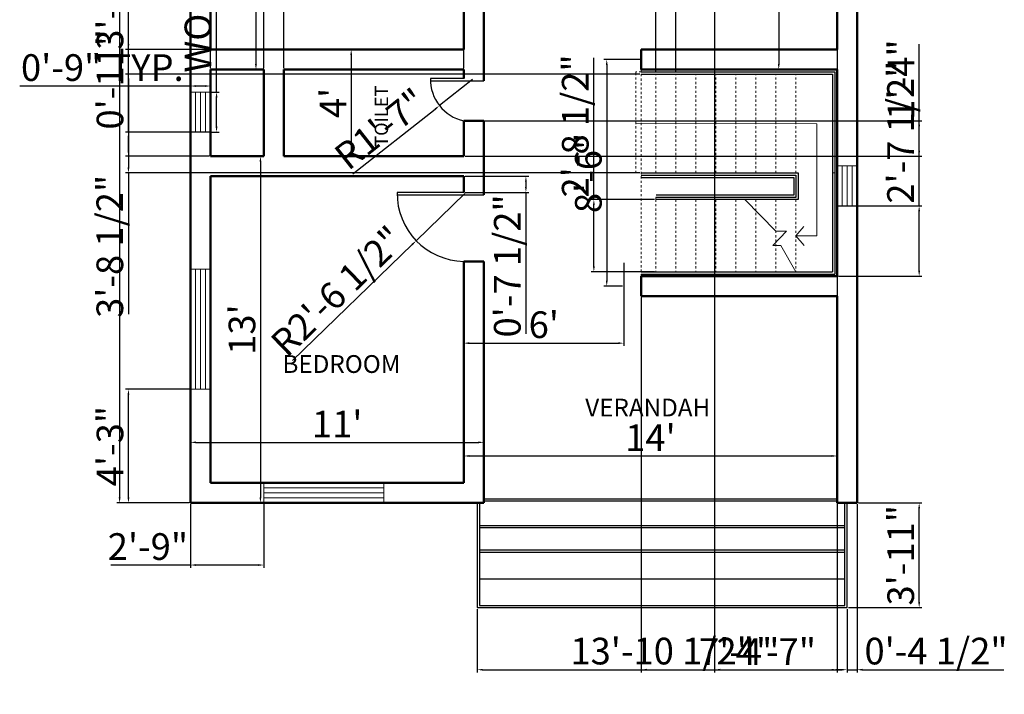
# Model space of a CAD drawing. Units: inches. Extents: x 2490 to 3058, y 1708 to 2351.
# Tile 1 of 2: x 2490 to 2933, y 1708 to 2012. Entities that reach past the tile are written whole.
import ezdxf

# ---------------------------------------------------------------- set-up
doc = ezdxf.new("R2010")
doc.units = ezdxf.units.IN
doc.linetypes.add('JIS_02_1.0', pattern=[2, 1, -1])
for name, color, linetype, lineweight in [('A-ANNO-DIMS', 2, 'Continuous', 18), ('A-ANNO-SYMB', 7, 'Continuous', 18), ('A-AREA-IDEN', 7, 'Continuous', 25), ('A-DOOR', 3, 'Continuous', 25), ('A-FLOR-STRS', 7, 'Continuous', 25), ('A-FLOR-STRS-OVHD', 8, 'JIS_02_1.0', 18), ('A-GLAZ', 4, 'Continuous', 18), ('A-WALL', 7, 'Continuous', 50)]:
    doc.layers.add(name, color=color, linetype=linetype, lineweight=lineweight)
doc.styles.get("Standard").update_dxf_attribs({"font": 'arial.ttf'})
doc.dimstyles.new('ISO-25', dxfattribs={"dimtxt": 12, "dimasz": 2.5, "dimexe": 1.25, "dimexo": 0.625, "dimtad": 1, "dimdec": 1, "dimlunit": 3, "dimtxsty": 'Standard', "dimcen": 2.5, "dimadec": 0, "dimazin": 0, "dimtfac": 1, "dimtdec": 1, "dimtmove": 0, "dimatfit": 3, "dimfxl": 1, "dimarcsym": 0})

# ---------------------------------------------------------------- blocks, each defined once
blk = doc.blocks.new('*D7')
at = {"layer": 'A-ANNO-DIMS', "color": 0, "lineweight": -2, "transparency": 16777216}
for p, q in [((2597.25, 2121.57), (2595.04, 2121.57)), ((2596.29, 2119.07), (2596.29, 1992.07)), ((2597.25, 1989.57), (2595.04, 1989.57))]:
    blk.add_line(p, q, dxfattribs=at)
at = {"layer": 'A-ANNO-DIMS', "color": 0, "transparency": 16777216}
for points in [[(2595.88, 2119.07), (2596.71, 2119.07), (2596.29, 2121.57)], [(2595.88, 1992.07), (2596.71, 1992.07), (2596.29, 1989.57)]]:
    blk.add_solid(points, dxfattribs=at)
at = {"layer": 'Defpoints', "color": 0, "transparency": 16777216}
for p in [(2597.88, 2121.57), (2596.29, 1989.57), (2597.88, 1989.57)]:
    blk.add_point(p, dxfattribs=at)
at = {"layer": 'A-ANNO-DIMS', "color": 0, "transparency": 16777216, "insert": (2589.64, 2055.57), "char_height": 12, "attachment_point": 5, "rotation": 90}
blk.add_mtext("11'", dxfattribs=at)
blk = doc.blocks.new('*D9')
at = {"layer": 'A-ANNO-DIMS', "color": 0, "lineweight": -2, "transparency": 16777216}
for p, q in [((2609.47, 1998.57), (2640.41, 1998.57)), ((2639.16, 1996.07), (2639.16, 1953.07)), ((2609.47, 1950.57), (2640.41, 1950.57))]:
    blk.add_line(p, q, dxfattribs=at)
at = {"layer": 'A-ANNO-DIMS', "color": 0, "transparency": 16777216}
for points in [[(2638.75, 1996.07), (2639.58, 1996.07), (2639.16, 1998.57)], [(2638.75, 1953.07), (2639.58, 1953.07), (2639.16, 1950.57)]]:
    blk.add_solid(points, dxfattribs=at)
at = {"layer": 'Defpoints', "color": 0, "transparency": 16777216}
for p in [(2608.85, 1998.57), (2608.85, 1950.57), (2639.16, 1950.57)]:
    blk.add_point(p, dxfattribs=at)
at = {"layer": 'A-ANNO-DIMS', "color": 0, "transparency": 16777216, "insert": (2632.54, 1974.57), "char_height": 12, "attachment_point": 5, "rotation": 90}
blk.add_mtext("4'", dxfattribs=at)
blk = doc.blocks.new('*D10')
at = {"layer": 'A-ANNO-DIMS', "color": 0, "lineweight": -2, "transparency": 16777216}
for p, q in [((2599.22, 1950.57), (2597.06, 1950.57)), ((2598.31, 1948.07), (2598.31, 1797.07)), ((2599.22, 1794.57), (2597.06, 1794.57))]:
    blk.add_line(p, q, dxfattribs=at)
at = {"layer": 'A-ANNO-DIMS', "color": 0, "transparency": 16777216}
for points in [[(2597.89, 1948.07), (2598.72, 1948.07), (2598.31, 1950.57)], [(2597.89, 1797.07), (2598.72, 1797.07), (2598.31, 1794.57)]]:
    blk.add_solid(points, dxfattribs=at)
at = {"layer": 'Defpoints', "color": 0, "transparency": 16777216}
for p in [(2599.85, 1950.57), (2598.31, 1794.57), (2599.85, 1794.57)]:
    blk.add_point(p, dxfattribs=at)
at = {"layer": 'A-ANNO-DIMS', "color": 0, "transparency": 16777216, "insert": (2591.55, 1872.57), "char_height": 12, "attachment_point": 5, "rotation": 90}
blk.add_mtext("13'", dxfattribs=at)
blk = doc.blocks.new('*D11')
at = {"layer": 'A-ANNO-DIMS', "color": 0, "lineweight": -2, "transparency": 16777216}
for p, q in [((2566.85, 1795.2), (2566.85, 1823.06)), ((2569.35, 1821.81), (2696.35, 1821.81)), ((2698.85, 1795.2), (2698.85, 1823.06))]:
    blk.add_line(p, q, dxfattribs=at)
at = {"layer": 'A-ANNO-DIMS', "color": 0, "transparency": 16777216}
for points in [[(2569.35, 1822.23), (2569.35, 1821.4), (2566.85, 1821.81)], [(2696.35, 1822.23), (2696.35, 1821.4), (2698.85, 1821.81)]]:
    blk.add_solid(points, dxfattribs=at)
at = {"layer": 'Defpoints', "color": 0, "transparency": 16777216}
for p in [(2698.85, 1821.81), (2566.85, 1794.57), (2698.85, 1794.57)]:
    blk.add_point(p, dxfattribs=at)
at = {"layer": 'A-ANNO-DIMS', "color": 0, "transparency": 16777216, "insert": (2632.85, 1828.46), "char_height": 12, "attachment_point": 5}
blk.add_mtext("11'", dxfattribs=at)
blk = doc.blocks.new('*D12')
at = {"layer": 'A-ANNO-DIMS', "color": 0, "lineweight": -2, "transparency": 16777216}
for p, q in [((2769.12, 1994.07), (2752.94, 1994.07)), ((2754.19, 1991.57), (2754.19, 1894.57)), ((2761.22, 1892.07), (2752.94, 1892.07))]:
    blk.add_line(p, q, dxfattribs=at)
at = {"layer": 'A-ANNO-DIMS', "color": 0, "transparency": 16777216}
for points in [[(2753.77, 1991.57), (2754.6, 1991.57), (2754.19, 1994.07)], [(2753.77, 1894.57), (2754.6, 1894.57), (2754.19, 1892.07)]]:
    blk.add_solid(points, dxfattribs=at)
at = {"layer": 'Defpoints', "color": 0, "transparency": 16777216}
for p in [(2769.74, 1994.07), (2754.19, 1892.07), (2761.85, 1892.07)]:
    blk.add_point(p, dxfattribs=at)
at = {"layer": 'A-ANNO-DIMS', "color": 0, "transparency": 16777216, "insert": (2747.43, 1943.07), "char_height": 12, "attachment_point": 5, "rotation": 90}
blk.add_mtext('8\'-6"', dxfattribs=at)
blk = doc.blocks.new('*D13')
at = {"layer": 'A-ANNO-DIMS', "color": 0, "lineweight": -2, "transparency": 16777216}
for p, q in [((2689.85, 1902.66), (2689.85, 1865.21)), ((2761.85, 1902.66), (2761.85, 1865.21)), ((2692.35, 1866.46), (2759.35, 1866.46))]:
    blk.add_line(p, q, dxfattribs=at)
at = {"layer": 'A-ANNO-DIMS', "color": 0, "transparency": 16777216}
for points in [[(2692.35, 1866.88), (2692.35, 1866.04), (2689.85, 1866.46)], [(2759.35, 1866.88), (2759.35, 1866.04), (2761.85, 1866.46)]]:
    blk.add_solid(points, dxfattribs=at)
at = {"layer": 'Defpoints', "color": 0, "transparency": 16777216}
for p in [(2689.85, 1903.28), (2761.85, 1903.28), (2761.85, 1866.46)]:
    blk.add_point(p, dxfattribs=at)
at = {"layer": 'A-ANNO-DIMS', "color": 0, "transparency": 16777216, "insert": (2725.85, 1873.21), "char_height": 12, "attachment_point": 5}
blk.add_mtext("6'", dxfattribs=at)
blk = doc.blocks.new('*D14')
at = {"layer": 'A-ANNO-DIMS', "color": 0, "lineweight": -2, "transparency": 16777216}
for p, q in [((2847.51, 2169.63), (2830.36, 2169.63)), ((2831.61, 2167.13), (2831.61, 1992.13)), ((2847.51, 1989.63), (2830.36, 1989.63))]:
    blk.add_line(p, q, dxfattribs=at)
at = {"layer": 'A-ANNO-DIMS', "color": 0, "transparency": 16777216}
for points in [[(2831.19, 2167.13), (2832.02, 2167.13), (2831.61, 2169.63)], [(2831.19, 1992.13), (2832.02, 1992.13), (2831.61, 1989.63)]]:
    blk.add_solid(points, dxfattribs=at)
at = {"layer": 'Defpoints', "color": 0, "transparency": 16777216}
for p in [(2848.13, 2169.63), (2831.61, 1989.63), (2848.13, 1989.63)]:
    blk.add_point(p, dxfattribs=at)
at = {"layer": 'A-ANNO-DIMS', "color": 0, "transparency": 16777216, "insert": (2824.86, 2079.63), "char_height": 12, "attachment_point": 5, "rotation": 90}
blk.add_mtext("15'", dxfattribs=at)
blk = doc.blocks.new('*D16')
at = {"layer": 'A-ANNO-DIMS', "color": 0, "lineweight": -2, "transparency": 16777216}
for p, q in [((2689.85, 1804.2), (2689.85, 1816.94)), ((2692.35, 1815.69), (2855.35, 1815.69)), ((2857.85, 1804.2), (2857.85, 1816.94))]:
    blk.add_line(p, q, dxfattribs=at)
at = {"layer": 'A-ANNO-DIMS', "color": 0, "transparency": 16777216}
for points in [[(2692.35, 1816.11), (2692.35, 1815.28), (2689.85, 1815.69)], [(2855.35, 1816.11), (2855.35, 1815.28), (2857.85, 1815.69)]]:
    blk.add_solid(points, dxfattribs=at)
at = {"layer": 'Defpoints', "color": 0, "transparency": 16777216}
for p in [(2857.85, 1815.69), (2689.85, 1803.57), (2857.85, 1803.57)]:
    blk.add_point(p, dxfattribs=at)
at = {"layer": 'A-ANNO-DIMS', "color": 0, "transparency": 16777216, "insert": (2773.85, 1822.34), "char_height": 12, "attachment_point": 5}
blk.add_mtext("14'", dxfattribs=at)
blk = doc.blocks.new('Window - Wood Frame 36 in. Wide plan')
for p, q in [((0, 6), (0, 0)), ((36, 6), (36, 0)), ((0, 4.5), (36, 4.5)), ((0, 3), (36, 3)), ((0, 1.5), (36, 1.5))]:
    blk.add_line(p, q)
blk = doc.blocks.new('*D22')
at = {"layer": 'A-ANNO-DIMS', "color": 0, "lineweight": -2, "transparency": 16777216}
for p, q in [((2566.22, 2274.57), (2533.68, 2274.57)), ((2534.93, 2272.07), (2534.93, 1797.07)), ((2566.22, 1794.57), (2533.68, 1794.57))]:
    blk.add_line(p, q, dxfattribs=at)
at = {"layer": 'A-ANNO-DIMS', "color": 0, "transparency": 16777216}
for points in [[(2534.51, 2272.07), (2535.35, 2272.07), (2534.93, 2274.57)], [(2534.51, 1797.07), (2535.35, 1797.07), (2534.93, 1794.57)]]:
    blk.add_solid(points, dxfattribs=at)
at = {"layer": 'Defpoints', "color": 0, "transparency": 16777216}
for p in [(2566.85, 2274.57), (2534.93, 1794.57), (2566.85, 1794.57)]:
    blk.add_point(p, dxfattribs=at)
at = {"layer": 'A-ANNO-DIMS', "color": 0, "transparency": 16777216, "insert": (2528.18, 2034.57), "char_height": 12, "attachment_point": 5, "rotation": 90}
blk.add_mtext("40'", dxfattribs=at)
blk = doc.blocks.new('*D26')
at = {"layer": 'A-ANNO-DIMS', "color": 0, "lineweight": -2, "transparency": 16777216}
for p, q in [((2578.55, 1979.48), (2578.55, 2193.75)), ((2576.47, 1979.48), (2579.8, 1979.48)), ((2578.55, 1963.98), (2578.55, 1976.98)), ((2576.47, 1961.48), (2579.8, 1961.48))]:
    blk.add_line(p, q, dxfattribs=at)
at = {"layer": 'A-ANNO-DIMS', "color": 0, "transparency": 16777216}
for points in [[(2578.13, 1976.98), (2578.97, 1976.98), (2578.55, 1979.48)], [(2578.13, 1963.98), (2578.97, 1963.98), (2578.55, 1961.48)]]:
    blk.add_solid(points, dxfattribs=at)
at = {"layer": 'Defpoints', "color": 0, "transparency": 16777216}
for p in [(2575.85, 1979.48), (2578.55, 1979.48), (2575.85, 1961.48)]:
    blk.add_point(p, dxfattribs=at)
at = {"layer": 'A-ANNO-DIMS', "color": 0, "transparency": 16777216, "insert": (2571.72, 2087.86), "char_height": 12, "attachment_point": 5, "rotation": 90}
blk.add_mtext('WOOD WINDOW 1\'-6" TYP.', dxfattribs=at)
blk = doc.blocks.new('*D27')
at = {"layer": 'A-ANNO-DIMS', "color": 0, "lineweight": -2, "transparency": 16777216}
for p, q in [((2566.85, 1982.18), (2489.95, 1982.18)), ((2566.85, 1980.11), (2566.85, 1983.43)), ((2573.35, 1982.18), (2569.35, 1982.18)), ((2575.85, 1980.11), (2575.85, 1983.43))]:
    blk.add_line(p, q, dxfattribs=at)
at = {"layer": 'A-ANNO-DIMS', "color": 0, "transparency": 16777216}
for points in [[(2569.35, 1982.6), (2569.35, 1981.76), (2566.85, 1982.18)], [(2573.35, 1982.6), (2573.35, 1981.76), (2575.85, 1982.18)]]:
    blk.add_solid(points, dxfattribs=at)
at = {"layer": 'Defpoints', "color": 0, "transparency": 16777216}
for p in [(2566.85, 1982.18), (2566.85, 1979.48), (2575.85, 1979.48)]:
    blk.add_point(p, dxfattribs=at)
at = {"layer": 'A-ANNO-DIMS', "color": 0, "transparency": 16777216, "insert": (2527.15, 1988.93), "char_height": 12, "attachment_point": 5}
blk.add_mtext('0\'-9" TYP.', dxfattribs=at)
blk = doc.blocks.new('*D30')
at = {"layer": 'A-ANNO-DIMS', "color": 0, "lineweight": -2, "transparency": 16777216}
for p, q in [((2695.91, 1746.82), (2695.91, 1718.25)), ((2862.35, 1746.82), (2862.35, 1718.25)), ((2698.41, 1719.5), (2859.85, 1719.5))]:
    blk.add_line(p, q, dxfattribs=at)
at = {"layer": 'A-ANNO-DIMS', "color": 0, "transparency": 16777216}
for points in [[(2698.41, 1719.92), (2698.41, 1719.08), (2695.91, 1719.5)], [(2859.85, 1719.92), (2859.85, 1719.08), (2862.35, 1719.5)]]:
    blk.add_solid(points, dxfattribs=at)
at = {"layer": 'Defpoints', "color": 0, "transparency": 16777216}
for p in [(2695.91, 1747.45), (2862.35, 1747.45), (2862.35, 1719.5)]:
    blk.add_point(p, dxfattribs=at)
at = {"layer": 'A-ANNO-DIMS', "color": 0, "transparency": 16777216, "insert": (2779.13, 1726.33), "char_height": 12, "attachment_point": 5}
blk.add_mtext('13\'-10 1/2"', dxfattribs=at)
blk = doc.blocks.new('*D31')
at = {"layer": 'A-ANNO-DIMS', "color": 0, "lineweight": -2, "transparency": 16777216}
for p, q in [((2867.47, 1794.57), (2896.05, 1794.57)), ((2894.8, 1749.95), (2894.8, 1792.07)), ((2862.97, 1747.45), (2896.05, 1747.45))]:
    blk.add_line(p, q, dxfattribs=at)
at = {"layer": 'A-ANNO-DIMS', "color": 0, "transparency": 16777216}
for points in [[(2894.38, 1792.07), (2895.22, 1792.07), (2894.8, 1794.57)], [(2894.38, 1749.95), (2895.22, 1749.95), (2894.8, 1747.45)]]:
    blk.add_solid(points, dxfattribs=at)
at = {"layer": 'Defpoints', "color": 0, "transparency": 16777216}
for p in [(2866.85, 1794.57), (2894.8, 1794.57), (2862.35, 1747.45)]:
    blk.add_point(p, dxfattribs=at)
at = {"layer": 'A-ANNO-DIMS', "color": 0, "transparency": 16777216, "insert": (2888.04, 1771.01), "char_height": 12, "attachment_point": 5, "rotation": 90}
blk.add_mtext('3\'-11"', dxfattribs=at)
blk = doc.blocks.new('*D32')
at = {"layer": 'A-ANNO-DIMS', "color": 0, "lineweight": -2, "transparency": 16777216}
for p, q in [((2769.74, 1886.95), (2769.74, 1718.25)), ((2857.85, 1886.95), (2857.85, 1718.25)), ((2772.24, 1719.5), (2855.35, 1719.5))]:
    blk.add_line(p, q, dxfattribs=at)
at = {"layer": 'A-ANNO-DIMS', "color": 0, "transparency": 16777216}
for points in [[(2772.24, 1719.92), (2772.24, 1719.08), (2769.74, 1719.5)], [(2855.35, 1719.92), (2855.35, 1719.08), (2857.85, 1719.5)]]:
    blk.add_solid(points, dxfattribs=at)
at = {"layer": 'Defpoints', "color": 0, "transparency": 16777216}
for p in [(2769.74, 1887.57), (2857.85, 1887.57), (2857.85, 1719.5)]:
    blk.add_point(p, dxfattribs=at)
at = {"layer": 'A-ANNO-DIMS', "color": 0, "transparency": 16777216, "insert": (2813.8, 1726.12), "char_height": 12, "attachment_point": 5}
blk.add_mtext('7\'-4"', dxfattribs=at)
blk = doc.blocks.new('*D33')
at = {"layer": 'A-ANNO-DIMS', "color": 0, "lineweight": -2, "transparency": 16777216}
for p, q in [((2608.85, 1990.2), (2608.85, 2303.77)), ((2611.35, 2302.52), (2687.35, 2302.52)), ((2689.85, 1990.2), (2689.85, 2303.77))]:
    blk.add_line(p, q, dxfattribs=at)
at = {"layer": 'A-ANNO-DIMS', "color": 0, "transparency": 16777216}
for points in [[(2611.35, 2302.94), (2611.35, 2302.1), (2608.85, 2302.52)], [(2687.35, 2302.94), (2687.35, 2302.1), (2689.85, 2302.52)]]:
    blk.add_solid(points, dxfattribs=at)
at = {"layer": 'Defpoints', "color": 0, "transparency": 16777216}
for p in [(2689.85, 2302.52), (2608.85, 1989.57), (2689.85, 1989.57)]:
    blk.add_point(p, dxfattribs=at)
at = {"layer": 'A-ANNO-DIMS', "color": 0, "transparency": 16777216, "insert": (2649.35, 2309.27), "char_height": 12, "attachment_point": 5}
blk.add_mtext('6\'-9"', dxfattribs=at)
blk = doc.blocks.new('*D36')
at = {"layer": 'A-ANNO-DIMS', "color": 0, "lineweight": -2, "transparency": 16777216}
for p, q in [((2802.74, 2168.95), (2802.74, 1718.25)), ((2857.85, 2168.95), (2857.85, 1718.25)), ((2805.24, 1719.5), (2855.35, 1719.5))]:
    blk.add_line(p, q, dxfattribs=at)
at = {"layer": 'A-ANNO-DIMS', "color": 0, "transparency": 16777216}
for points in [[(2805.24, 1719.92), (2805.24, 1719.08), (2802.74, 1719.5)], [(2855.35, 1719.92), (2855.35, 1719.08), (2857.85, 1719.5)]]:
    blk.add_solid(points, dxfattribs=at)
at = {"layer": 'Defpoints', "color": 0, "transparency": 16777216}
for p in [(2802.74, 2169.57), (2857.85, 2169.57), (2857.85, 1719.5)]:
    blk.add_point(p, dxfattribs=at)
at = {"layer": 'A-ANNO-DIMS', "color": 0, "transparency": 16777216, "insert": (2830.3, 1726.12), "char_height": 12, "attachment_point": 5}
blk.add_mtext('4\'-7"', dxfattribs=at)
blk = doc.blocks.new('*D38')
at = {"layer": 'A-ANNO-DIMS', "color": 0, "lineweight": -2, "transparency": 16777216}
for p, q in [((2894.8, 1966.57), (2894.8, 2001.09)), ((2690.47, 1966.57), (2896.05, 1966.57)), ((2894.8, 1953.07), (2894.8, 1964.07)), ((2690.47, 1950.57), (2896.05, 1950.57))]:
    blk.add_line(p, q, dxfattribs=at)
at = {"layer": 'A-ANNO-DIMS', "color": 0, "transparency": 16777216}
for points in [[(2894.38, 1964.07), (2895.22, 1964.07), (2894.8, 1966.57)], [(2894.38, 1953.07), (2895.22, 1953.07), (2894.8, 1950.57)]]:
    blk.add_solid(points, dxfattribs=at)
at = {"layer": 'Defpoints', "color": 0, "transparency": 16777216}
for p in [(2689.85, 1966.57), (2894.8, 1966.57), (2689.85, 1950.57)]:
    blk.add_point(p, dxfattribs=at)
at = {"layer": 'A-ANNO-DIMS', "color": 0, "transparency": 16777216, "insert": (2888.15, 1985.08), "char_height": 12, "attachment_point": 5, "rotation": 90}
blk.add_mtext('1\'-4"', dxfattribs=at)
blk = doc.blocks.new('*D39')
at = {"layer": 'A-ANNO-DIMS', "color": 0, "lineweight": -2, "transparency": 16777216}
for p, q in [((2538.9, 1961.48), (2538.9, 2006.45)), ((2575.22, 1961.48), (2537.65, 1961.48)), ((2538.9, 1953.07), (2538.9, 1958.98)), ((2575.22, 1950.57), (2537.65, 1950.57))]:
    blk.add_line(p, q, dxfattribs=at)
at = {"layer": 'A-ANNO-DIMS', "color": 0, "transparency": 16777216}
for points in [[(2538.48, 1958.98), (2539.32, 1958.98), (2538.9, 1961.48)], [(2538.48, 1953.07), (2539.32, 1953.07), (2538.9, 1950.57)]]:
    blk.add_solid(points, dxfattribs=at)
at = {"layer": 'Defpoints', "color": 0, "transparency": 16777216}
for p in [(2538.9, 1961.48), (2575.85, 1961.48), (2575.85, 1950.57)]:
    blk.add_point(p, dxfattribs=at)
at = {"layer": 'A-ANNO-DIMS', "color": 0, "transparency": 16777216, "insert": (2532.15, 1985.22), "char_height": 12, "attachment_point": 5, "rotation": 90}
blk.add_mtext('0\'-11"', dxfattribs=at)
blk = doc.blocks.new('*D40')
at = {"layer": 'A-ANNO-DIMS', "color": 0, "lineweight": -2, "transparency": 16777216}
for p, q in [((2575.85, 1990.2), (2575.85, 2303.77)), ((2578.35, 2302.52), (2597.35, 2302.52)), ((2599.85, 1990.2), (2599.85, 2303.77)), ((2599.85, 2302.52), (2635.7, 2302.52))]:
    blk.add_line(p, q, dxfattribs=at)
at = {"layer": 'A-ANNO-DIMS', "color": 0, "transparency": 16777216}
for points in [[(2578.35, 2302.94), (2578.35, 2302.1), (2575.85, 2302.52)], [(2597.35, 2302.94), (2597.35, 2302.1), (2599.85, 2302.52)]]:
    blk.add_solid(points, dxfattribs=at)
at = {"layer": 'Defpoints', "color": 0, "transparency": 16777216}
for p in [(2599.85, 2302.52), (2575.85, 1989.57), (2599.85, 1989.57)]:
    blk.add_point(p, dxfattribs=at)
at = {"layer": 'A-ANNO-DIMS', "color": 0, "transparency": 16777216, "insert": (2619.03, 2309.27), "char_height": 12, "attachment_point": 5}
blk.add_mtext('2\'-0"', dxfattribs=at)
blk = doc.blocks.new('*D43')
at = {"layer": 'A-ANNO-DIMS', "color": 0, "lineweight": -2, "transparency": 16777216}
for p, q in [((2575.22, 2034.57), (2537.65, 2034.57)), ((2538.9, 2001.07), (2538.9, 2032.07)), ((2575.22, 1998.57), (2537.65, 1998.57))]:
    blk.add_line(p, q, dxfattribs=at)
at = {"layer": 'A-ANNO-DIMS', "color": 0, "transparency": 16777216}
for points in [[(2538.48, 2032.07), (2539.32, 2032.07), (2538.9, 2034.57)], [(2538.48, 2001.07), (2539.32, 2001.07), (2538.9, 1998.57)]]:
    blk.add_solid(points, dxfattribs=at)
at = {"layer": 'Defpoints', "color": 0, "transparency": 16777216}
for p in [(2538.9, 2034.57), (2575.85, 2034.57), (2575.85, 1998.57)]:
    blk.add_point(p, dxfattribs=at)
at = {"layer": 'A-ANNO-DIMS', "color": 0, "transparency": 16777216, "insert": (2532.14, 2016.57), "char_height": 12, "attachment_point": 5, "rotation": 90}
blk.add_mtext('3\'-0"', dxfattribs=at)
blk = doc.blocks.new('*D44')
at = {"layer": 'A-ANNO-DIMS', "color": 0, "lineweight": -2, "transparency": 16777216}
for p, q in [((2566.22, 1845.71), (2537.65, 1845.71)), ((2538.9, 1797.07), (2538.9, 1843.21)), ((2566.22, 1794.57), (2537.65, 1794.57))]:
    blk.add_line(p, q, dxfattribs=at)
at = {"layer": 'A-ANNO-DIMS', "color": 0, "transparency": 16777216}
for points in [[(2538.48, 1843.21), (2539.32, 1843.21), (2538.9, 1845.71)], [(2538.48, 1797.07), (2539.32, 1797.07), (2538.9, 1794.57)]]:
    blk.add_solid(points, dxfattribs=at)
at = {"layer": 'Defpoints', "color": 0, "transparency": 16777216}
for p in [(2538.9, 1845.71), (2566.85, 1845.71), (2566.85, 1794.57)]:
    blk.add_point(p, dxfattribs=at)
at = {"layer": 'A-ANNO-DIMS', "color": 0, "transparency": 16777216, "insert": (2532.14, 1820.14), "char_height": 12, "attachment_point": 5, "rotation": 90}
blk.add_mtext('4\'-3"', dxfattribs=at)
blk = doc.blocks.new('*D45')
at = {"layer": 'A-ANNO-DIMS', "color": 0, "lineweight": -2, "transparency": 16777216}
for p, q in [((2566.85, 1793.95), (2566.85, 1765.37)), ((2599.85, 1793.95), (2599.85, 1765.37)), ((2566.85, 1766.62), (2531, 1766.62)), ((2597.35, 1766.62), (2569.35, 1766.62))]:
    blk.add_line(p, q, dxfattribs=at)
at = {"layer": 'A-ANNO-DIMS', "color": 0, "transparency": 16777216}
for points in [[(2569.35, 1767.04), (2569.35, 1766.2), (2566.85, 1766.62)], [(2597.35, 1767.04), (2597.35, 1766.2), (2599.85, 1766.62)]]:
    blk.add_solid(points, dxfattribs=at)
at = {"layer": 'Defpoints', "color": 0, "transparency": 16777216}
for p in [(2566.85, 1794.57), (2599.85, 1794.57), (2566.85, 1766.62)]:
    blk.add_point(p, dxfattribs=at)
at = {"layer": 'A-ANNO-DIMS', "color": 0, "transparency": 16777216, "insert": (2547.67, 1773.37), "char_height": 12, "attachment_point": 5}
blk.add_mtext('2\'-9"', dxfattribs=at)
blk = doc.blocks.new('*D47')
at = {"layer": 'A-ANNO-DIMS', "color": 0, "lineweight": -2, "transparency": 16777216}
for p, q in [((2894.8, 1928.26), (2894.8, 1992.08)), ((2858.47, 1928.26), (2896.05, 1928.26)), ((2894.8, 1899.07), (2894.8, 1925.76)), ((2858.47, 1896.57), (2896.05, 1896.57))]:
    blk.add_line(p, q, dxfattribs=at)
at = {"layer": 'A-ANNO-DIMS', "color": 0, "transparency": 16777216}
for points in [[(2894.38, 1925.76), (2895.22, 1925.76), (2894.8, 1928.26)], [(2894.38, 1899.07), (2895.22, 1899.07), (2894.8, 1896.57)]]:
    blk.add_solid(points, dxfattribs=at)
at = {"layer": 'Defpoints', "color": 0, "transparency": 16777216}
for p in [(2857.85, 1928.26), (2894.8, 1928.26), (2857.85, 1896.57)]:
    blk.add_point(p, dxfattribs=at)
at = {"layer": 'A-ANNO-DIMS', "color": 0, "transparency": 16777216, "insert": (2887.97, 1961.42), "char_height": 12, "attachment_point": 5, "rotation": 90}
blk.add_mtext('2\'-7 1/2"', dxfattribs=at)
blk = doc.blocks.new('*D50')
at = {"layer": 'A-ANNO-DIMS', "color": 0, "lineweight": -2, "transparency": 16777216}
for p, q in [((2690.47, 1941.57), (2719.05, 1941.57)), ((2717.8, 1939.07), (2717.8, 1936.78)), ((2690.47, 1934.28), (2719.05, 1934.28)), ((2717.8, 1934.28), (2717.8, 1870.67))]:
    blk.add_line(p, q, dxfattribs=at)
at = {"layer": 'A-ANNO-DIMS', "color": 0, "transparency": 16777216}
for points in [[(2717.38, 1939.07), (2718.22, 1939.07), (2717.8, 1941.57)], [(2717.38, 1936.78), (2718.22, 1936.78), (2717.8, 1934.28)]]:
    blk.add_solid(points, dxfattribs=at)
at = {"layer": 'Defpoints', "color": 0, "transparency": 16777216}
for p in [(2689.85, 1941.57), (2689.85, 1934.28), (2717.8, 1934.28)]:
    blk.add_point(p, dxfattribs=at)
at = {"layer": 'A-ANNO-DIMS', "color": 0, "transparency": 16777216, "insert": (2710.97, 1901.23), "char_height": 12, "attachment_point": 5, "rotation": 90}
blk.add_mtext('0\'-7 1/2"', dxfattribs=at)
blk = doc.blocks.new('*D51')
at = {"layer": 'A-ANNO-DIMS', "color": 0, "lineweight": -2, "transparency": 16777216}
for p, q in [((2776.33, 1988.2), (2776.33, 2303.77)), ((2778.83, 2302.52), (2782.83, 2302.52)), ((2785.33, 1988.2), (2785.33, 2303.77)), ((2785.33, 2302.52), (2820.98, 2302.52))]:
    blk.add_line(p, q, dxfattribs=at)
at = {"layer": 'A-ANNO-DIMS', "color": 0, "transparency": 16777216}
for points in [[(2778.83, 2302.94), (2778.83, 2302.1), (2776.33, 2302.52)], [(2782.83, 2302.94), (2782.83, 2302.1), (2785.33, 2302.52)]]:
    blk.add_solid(points, dxfattribs=at)
at = {"layer": 'Defpoints', "color": 0, "transparency": 16777216}
for p in [(2785.33, 2302.52), (2776.33, 1987.57), (2785.33, 1987.57)]:
    blk.add_point(p, dxfattribs=at)
at = {"layer": 'A-ANNO-DIMS', "color": 0, "transparency": 16777216, "insert": (2804.41, 2309.27), "char_height": 12, "attachment_point": 5}
blk.add_mtext('0\'-9"', dxfattribs=at)
blk = doc.blocks.new('*D52')
at = {"layer": 'A-ANNO-DIMS', "color": 0, "lineweight": -2, "transparency": 16777216}
for p, q in [((2769.12, 1987.57), (2537.65, 1987.57)), ((2538.9, 1985.07), (2538.9, 1945.57)), ((2769.12, 1943.07), (2537.65, 1943.07)), ((2538.9, 1943.07), (2538.9, 1879.47))]:
    blk.add_line(p, q, dxfattribs=at)
at = {"layer": 'A-ANNO-DIMS', "color": 0, "transparency": 16777216}
for points in [[(2538.48, 1985.07), (2539.32, 1985.07), (2538.9, 1987.57)], [(2538.48, 1945.57), (2539.32, 1945.57), (2538.9, 1943.07)]]:
    blk.add_solid(points, dxfattribs=at)
at = {"layer": 'Defpoints', "color": 0, "transparency": 16777216}
for p in [(2769.74, 1987.57), (2538.9, 1943.07), (2769.74, 1943.07)]:
    blk.add_point(p, dxfattribs=at)
at = {"layer": 'A-ANNO-DIMS', "color": 0, "transparency": 16777216, "insert": (2532.07, 1910.02), "char_height": 12, "attachment_point": 5, "rotation": 90}
blk.add_mtext('3\'-8 1/2"', dxfattribs=at)
blk = doc.blocks.new('*D53')
at = {"layer": 'A-ANNO-DIMS', "color": 0, "lineweight": -2, "transparency": 16777216}
for p, q in [((2748.38, 1931.07), (2748.38, 1994.89)), ((2775.71, 1931.07), (2747.13, 1931.07)), ((2748.38, 1901.07), (2748.38, 1928.57)), ((2775.71, 1898.57), (2747.13, 1898.57))]:
    blk.add_line(p, q, dxfattribs=at)
at = {"layer": 'A-ANNO-DIMS', "color": 0, "transparency": 16777216}
for points in [[(2747.96, 1928.57), (2748.8, 1928.57), (2748.38, 1931.07)], [(2747.96, 1901.07), (2748.8, 1901.07), (2748.38, 1898.57)]]:
    blk.add_solid(points, dxfattribs=at)
at = {"layer": 'Defpoints', "color": 0, "transparency": 16777216}
for p in [(2748.38, 1931.07), (2776.33, 1931.07), (2776.33, 1898.57)]:
    blk.add_point(p, dxfattribs=at)
at = {"layer": 'A-ANNO-DIMS', "color": 0, "transparency": 16777216, "insert": (2741.55, 1964.23), "char_height": 12, "attachment_point": 5, "rotation": 90}
blk.add_mtext('2\'-8 1/2"', dxfattribs=at)
blk = doc.blocks.new('*D54')
at = {"layer": 'A-ANNO-DIMS', "color": 0, "lineweight": -2, "transparency": 16777216}
for p, q in [((2866.85, 1793.95), (2866.85, 1718.25)), ((2862.35, 1746.82), (2862.35, 1718.25)), ((2859.85, 1719.5), (2857.35, 1719.5)), ((2862.35, 1719.5), (2866.85, 1719.5)), ((2869.35, 1719.5), (2932.96, 1719.5))]:
    blk.add_line(p, q, dxfattribs=at)
at = {"layer": 'A-ANNO-DIMS', "color": 0, "transparency": 16777216}
for points in [[(2859.85, 1719.92), (2859.85, 1719.08), (2862.35, 1719.5)], [(2869.35, 1719.92), (2869.35, 1719.08), (2866.85, 1719.5)]]:
    blk.add_solid(points, dxfattribs=at)
at = {"layer": 'Defpoints', "color": 0, "transparency": 16777216}
for p in [(2866.85, 1794.57), (2862.35, 1747.45), (2866.85, 1719.5)]:
    blk.add_point(p, dxfattribs=at)
at = {"layer": 'A-ANNO-DIMS', "color": 0, "transparency": 16777216, "insert": (2902.4, 1726.33), "char_height": 12, "attachment_point": 5}
blk.add_mtext('0\'-4 1/2"', dxfattribs=at)
blk = doc.blocks.new('*D55')
at = {"layer": 'A-ANNO-DIMS', "color": 0, "lineweight": -2, "transparency": 16777216}
for p, q in [((2690.35, 1933.78), (2668.43, 1912.57)), ((2612.67, 1858.61), (2666.63, 1910.83))]:
    blk.add_line(p, q, dxfattribs=at)
at = {"layer": 'A-ANNO-DIMS', "color": 0, "transparency": 16777216}
blk.add_solid([(2666.34, 1911.13), (2666.92, 1910.53), (2668.43, 1912.57)], dxfattribs=at)
at = {"layer": 'Defpoints', "color": 0, "transparency": 16777216}
for p in [(2690.35, 1933.78), (2668.43, 1912.57)]:
    blk.add_point(p, dxfattribs=at)
at = {"layer": 'A-ANNO-DIMS', "color": 0, "transparency": 16777216, "insert": (2634, 1888.76), "char_height": 12, "attachment_point": 5, "rotation": 44.0613}
blk.add_mtext('R2\'-6 1/2"', dxfattribs=at)
blk = doc.blocks.new('*D60')
at = {"layer": 'A-ANNO-DIMS', "color": 0, "lineweight": -2, "transparency": 16777216}
for p, q in [((2693.75, 1985.07), (2678.91, 1973.36)), ((2639.95, 1942.6), (2676.95, 1971.81))]:
    blk.add_line(p, q, dxfattribs=at)
at = {"layer": 'A-ANNO-DIMS', "color": 0, "transparency": 16777216}
blk.add_solid([(2676.69, 1972.13), (2677.21, 1971.48), (2678.91, 1973.36)], dxfattribs=at)
at = {"layer": 'Defpoints', "color": 0, "transparency": 16777216}
for p in [(2693.75, 1985.07), (2678.91, 1973.36)]:
    blk.add_point(p, dxfattribs=at)
at = {"layer": 'A-ANNO-DIMS', "color": 0, "transparency": 16777216, "insert": (2653.35, 1961.65), "char_height": 12, "attachment_point": 5, "rotation": 38.2892}
blk.add_mtext('R1\'-7"', dxfattribs=at)

msp = doc.modelspace()

# ---------------------------------------------------------------- linework, layer by layer
at = {"layer": 'A-ANNO-SYMB'}
for p, q in [((2767.33, 1965.32), (2848.7, 1965.11)), ((2848.7, 1965.11), (2848.7, 1914.82)), ((2830.33, 1916.81), (2816.33, 1931.07)), ((2828.89, 1910.43), (2835.07, 1916.81)), ((2835.07, 1916.81), (2830.33, 1916.81)), ((2839.33, 1914.82), (2842.85, 1918.92)), ((2848.7, 1914.82), (2839.33, 1914.82)), ((2839.33, 1914.82), (2842.98, 1910.36)), ((2832.49, 1910.43), (2828.89, 1910.43)), ((2839.33, 1898.57), (2832.49, 1910.43))]:
    msp.add_line(p, q, dxfattribs=at)
at = {"layer": 'A-DOOR'}
for p, q in [((2689.85, 1985.57), (2674.85, 1985.57)), ((2674.85, 1985.57), (2674.85, 1984.57)), ((2674.85, 1984.57), (2698.85, 1984.57)), ((2689.85, 1934.28), (2659.85, 1934.28)), ((2659.85, 1934.28), (2659.85, 1933.28)), ((2659.85, 1933.28), (2698.85, 1933.28))]:
    msp.add_line(p, q, dxfattribs=at)
for centre, radius, start, end in [((2693.75, 1985.07), 18.91, 178.4846, 258.0957), ((2690.35, 1933.78), 30.5, 179.0608, 269.0608)]:
    msp.add_arc(centre, radius, start, end, dxfattribs=at)
at = {"layer": 'A-FLOR-STRS'}
for p, q in [((2769.74, 1988.57), (2856.85, 1988.57)), ((2769.74, 1987.57), (2855.85, 1987.57)), ((2855.85, 1987.57), (2855.85, 1898.57)), ((2856.85, 1988.57), (2856.85, 1897.57)), ((2769.74, 1943.07), (2840.33, 1943.07)), ((2769.74, 1942.07), (2839.33, 1942.07)), ((2839.33, 1942.07), (2839.33, 1932.07)), ((2840.33, 1943.07), (2840.33, 1931.07)), ((2769.74, 1941.07), (2838.33, 1941.07)), ((2838.33, 1941.07), (2838.33, 1933.07)), ((2838.33, 1933.07), (2776.5, 1933.07)), ((2839.33, 1932.07), (2776.33, 1932.07)), ((2840.33, 1931.07), (2776.33, 1931.07)), ((2769.74, 1898.57), (2855.85, 1898.57)), ((2769.74, 1897.57), (2856.85, 1897.57)), ((2698.85, 1796.45), (2857.85, 1796.45)), ((2698.85, 1795.45), (2857.85, 1795.45)), ((2695.91, 1794.57), (2695.91, 1747.45)), ((2696.91, 1794.57), (2696.91, 1748.45)), ((2861.35, 1748.45), (2861.35, 1794.57)), ((2862.35, 1747.45), (2862.35, 1794.57)), ((2696.91, 1784.45), (2861.35, 1784.45)), ((2696.91, 1783.45), (2861.35, 1783.45)), ((2696.91, 1773.45), (2861.35, 1773.45)), ((2696.91, 1772.45), (2861.35, 1772.45)), ((2696.91, 1760.45), (2861.35, 1760.45)), ((2695.91, 1747.45), (2862.35, 1747.45)), ((2696.91, 1748.45), (2861.35, 1748.45))]:
    msp.add_line(p, q, dxfattribs=at)
at = {"layer": 'A-FLOR-STRS-OVHD'}
for p, q in [((2769.74, 1988.57), (2767.33, 1988.57)), ((2767.33, 1988.57), (2767.33, 1987.57)), ((2767.33, 1943.07), (2767.33, 1987.57)), ((2769.74, 1989.57), (2769.74, 1896.57)), ((2776.33, 1943.07), (2776.33, 1987.57)), ((2785.33, 1943.07), (2785.33, 1987.57)), ((2794.33, 1943.07), (2794.33, 1987.57)), ((2803.33, 1943.07), (2803.33, 1987.57)), ((2812.33, 1943.07), (2812.33, 1987.57)), ((2821.33, 1943.07), (2821.33, 1987.57)), ((2830.33, 1943.07), (2830.33, 1987.57)), ((2839.33, 1943.07), (2839.33, 1987.57)), ((2769.74, 1896.57), (2769.74, 1943.07)), ((2769.74, 1943.07), (2840.33, 1943.07)), ((2855.85, 1943.07), (2857.85, 1943.07)), ((2779.47, 1933.07), (2776.33, 1933.07)), ((2776.33, 1931.07), (2776.33, 1933.07)), ((2776.33, 1931.07), (2776.33, 1898.57)), ((2785.33, 1931.07), (2785.33, 1898.57)), ((2794.33, 1931.07), (2794.33, 1898.57)), ((2803.33, 1931.07), (2803.33, 1898.57)), ((2812.33, 1931.07), (2812.33, 1898.57)), ((2821.33, 1931.07), (2821.33, 1898.57)), ((2830.33, 1931.07), (2830.33, 1898.57)), ((2839.33, 1930.36), (2839.33, 1931.07)), ((2839.33, 1931.07), (2839.33, 1898.57))]:
    msp.add_line(p, q, dxfattribs=at)
at = {"layer": 'A-WALL'}
for p, q in [((2566.85, 1794.57), (2566.85, 2274.57)), ((2866.85, 2274.57), (2866.85, 1794.57)), ((2575.85, 1998.57), (2575.85, 2265.57)), ((2857.85, 2169.57), (2857.85, 1998.57)), ((2689.85, 1998.57), (2689.85, 2092.42)), ((2698.85, 1984.57), (2698.85, 2092.42)), ((2575.85, 1998.57), (2689.85, 1998.57)), ((2769.74, 1998.57), (2857.85, 1998.57)), ((2769.74, 1998.57), (2769.74, 1989.57)), ((2575.85, 1989.57), (2599.85, 1989.57)), ((2575.85, 1989.57), (2599.85, 1989.57)), ((2575.85, 1950.57), (2575.85, 1989.57)), ((2599.85, 1989.57), (2599.85, 1950.57)), ((2608.85, 1950.57), (2608.85, 1989.57)), ((2608.85, 1989.57), (2689.85, 1989.57)), ((2689.85, 1985.57), (2689.85, 1989.57)), ((2698.85, 1989.57), (2698.85, 1988.57)), ((2698.85, 1988.57), (2698.85, 1985.57)), ((2769.74, 1989.57), (2857.85, 1989.57)), ((2857.85, 1989.57), (2857.85, 1896.57)), ((2689.85, 1966.57), (2698.85, 1966.57)), ((2689.85, 1950.57), (2689.85, 1966.57)), ((2698.85, 1966.57), (2698.85, 1960.57)), ((2698.85, 1933.28), (2698.85, 1966.57)), ((2575.85, 1950.57), (2599.85, 1950.57)), ((2608.85, 1950.57), (2689.85, 1950.57)), ((2575.85, 1803.57), (2575.85, 1941.57)), ((2575.85, 1941.57), (2689.85, 1941.57)), ((2689.85, 1934.28), (2689.85, 1941.57)), ((2689.85, 1803.57), (2689.85, 1903.28)), ((2698.85, 1903.28), (2689.85, 1903.28)), ((2698.85, 1794.57), (2698.85, 1903.28)), ((2769.74, 1896.57), (2857.85, 1896.57)), ((2769.74, 1896.57), (2769.74, 1887.57)), ((2769.74, 1887.57), (2857.85, 1887.57)), ((2857.85, 1887.57), (2857.85, 1794.57)), ((2689.85, 1803.57), (2575.85, 1803.57)), ((2857.85, 1799.24), (2857.85, 1800.24)), ((2698.85, 1794.57), (2566.85, 1794.57)), ((2866.85, 1794.57), (2857.85, 1794.57))]:
    msp.add_line(p, q, dxfattribs=at)

# ---------------------------------------------------------------- block references
at = {"layer": 'A-GLAZ', "yscale": 1.5, "rotation": 90}
for p, xscale in [((2575.85, 1961.48), 0.5), ((2866.85, 1928.26), 0.5), ((2575.85, 1845.71), 1.5)]:
    msp.add_blockref('Window - Wood Frame 36 in. Wide plan', p, dxfattribs=dict(at, xscale=xscale))
at = {"layer": 'A-GLAZ', "xscale": 1.5, "yscale": 1.5}
msp.add_blockref('Window - Wood Frame 36 in. Wide plan', (2599.85, 1794.57), dxfattribs=at)

# ---------------------------------------------------------------- texts
at = {"layer": 'A-AREA-IDEN', "insert": (2649.78, 1954.84), "char_height": 6, "attachment_point": 1, "rotation": 90}
msp.add_mtext_dynamic_manual_height_columns('TOILET', width=31.2754, gutter_width=12.5, heights=[0], dxfattribs=at)
at = {"layer": 'A-AREA-IDEN', "char_height": 8, "attachment_point": 1}
for s, width, insert in [('BEDROOM', 0.8182, (2608.23, 1861.07)), ('VERANDAH', 84.6482, (2744.51, 1841.48))]:
    msp.add_mtext_dynamic_manual_height_columns(s, width=width, gutter_width=12.5, heights=[0], dxfattribs=dict(at, insert=insert))

# ---------------------------------------------------------------- dimensions: what is measured, and where the dimension line sits
at = {"layer": 'A-ANNO-DIMS'}
for base, p1, p2, override, picture, middle in [((2599.85, 2302.52), (2575.85, 1989.57), (2599.85, 1989.57), {"dimdec": 1, "dimlfac": 1, "dimrnd": 0, "dimzin": 1, "dimdsep": 46, "dimlunit": 4, "dimfrac": 2}, '*D40', (2619.03, 2309.27)), ((2689.85, 2302.52), (2608.85, 1989.57), (2689.85, 1989.57), {"dimdec": 1, "dimlfac": 1, "dimrnd": 0, "dimzin": 1, "dimdsep": 46, "dimlunit": 4, "dimfrac": 2}, '*D33', (2649.35, 2309.27)), ((2785.33, 2302.52), (2776.33, 1987.57), (2785.33, 1987.57), {"dimdec": 1, "dimlfac": 1, "dimrnd": 0, "dimzin": 1, "dimdsep": 46, "dimlunit": 4, "dimfrac": 2}, '*D51', (2804.41, 2309.27)), ((2857.85, 1719.5), (2802.74, 2169.57), (2857.85, 2169.57), {"dimdec": 1, "dimlfac": 1, "dimrnd": 0, "dimzin": 1, "dimdsep": 46, "dimlunit": 4, "dimfrac": 2}, '*D36', (2830.3, 1726.12)), ((2761.85, 1866.46), (2689.85, 1903.28), (2761.85, 1903.28), {"dimclrd": 0, "dimclre": 0, "dimclrt": 0}, '*D13', (2725.85, 1873.21)), ((2857.85, 1719.5), (2769.74, 1887.57), (2857.85, 1887.57), {"dimdec": 1, "dimlfac": 1, "dimrnd": 0, "dimzin": 1, "dimdsep": 46, "dimlunit": 4, "dimfrac": 2}, '*D32', (2813.8, 1726.12)), ((2698.85, 1821.81), (2566.85, 1794.57), (2698.85, 1794.57), {"dimclrd": 0, "dimclre": 0, "dimclrt": 0}, '*D11', (2632.85, 1828.46)), ((2857.85, 1815.69), (2689.85, 1803.57), (2857.85, 1803.57), {"dimclrd": 0, "dimclre": 0, "dimclrt": 0}, '*D16', (2773.85, 1822.34)), ((2866.85, 1719.5), (2862.35, 1747.45), (2866.85, 1794.57), {"dimdec": 1, "dimlfac": 1, "dimrnd": 0, "dimzin": 1, "dimdsep": 46, "dimlunit": 4, "dimfrac": 2}, '*D54', (2902.4, 1726.33)), ((2862.35, 1719.5), (2695.91, 1747.45), (2862.35, 1747.45), {"dimdec": 1, "dimlfac": 1, "dimrnd": 0, "dimzin": 1, "dimdsep": 46, "dimlunit": 4, "dimfrac": 2}, '*D30', (2779.13, 1726.33))]:
    dim = msp.add_linear_dim(base=base, p1=p1, p2=p2, dimstyle='ISO-25', override=override, dxfattribs=at)
    dim.commit()
    dim.dimension.update_dxf_attribs({"geometry": picture, "text_midpoint": middle})
for base, p1, p2, angle, override, picture, middle in [((2534.93, 1794.57), (2566.85, 2274.57), (2566.85, 1794.57), 90, {"dimclrd": 0, "dimclre": 0, "dimclrt": 0}, '*D22', (2528.18, 2034.57)), ((2596.29, 1989.57), (2597.88, 2121.57), (2597.88, 1989.57), 90, {"dimclrd": 0, "dimclre": 0, "dimclrt": 0}, '*D7', (2589.64, 2055.57)), ((2538.9, 2034.57), (2575.85, 1998.57), (2575.85, 2034.57), 90, {"dimdec": 1, "dimlfac": 1, "dimrnd": 0, "dimzin": 1, "dimdsep": 46, "dimlunit": 4, "dimfrac": 2}, '*D43', (2532.14, 2016.57)), ((2538.9, 1961.48), (2575.85, 1950.57), (2575.85, 1961.48), 90, {"dimdec": 1, "dimlfac": 1, "dimrnd": 0, "dimzin": 1, "dimdsep": 46, "dimlunit": 4, "dimfrac": 2}, '*D39', (2532.15, 1985.22)), ((2894.8, 1966.57), (2689.85, 1950.57), (2689.85, 1966.57), 90, {"dimdec": 1, "dimlfac": 1, "dimrnd": 0, "dimzin": 1, "dimdsep": 46, "dimlunit": 4, "dimfrac": 2}, '*D38', (2888.15, 1985.08)), ((2639.16, 1950.57), (2608.85, 1998.57), (2608.85, 1950.57), 90, {"dimclrd": 0, "dimclre": 0, "dimclrt": 0}, '*D9', (2632.54, 1974.57)), ((2748.38, 1931.07), (2776.33, 1898.57), (2776.33, 1931.07), 90, {"dimdec": 1, "dimlfac": 1, "dimrnd": 0, "dimzin": 1, "dimdsep": 46, "dimlunit": 4, "dimfrac": 2}, '*D53', (2741.55, 1964.23)), ((2754.19, 1892.07), (2769.74, 1994.07), (2761.85, 1892.07), 90, {"dimclrd": 0, "dimclre": 0, "dimclrt": 0}, '*D12', (2747.43, 1943.07)), ((2894.8, 1928.26), (2857.85, 1896.57), (2857.85, 1928.26), 90, {"dimdec": 1, "dimlfac": 1, "dimrnd": 0, "dimzin": 1, "dimdsep": 46, "dimlunit": 4, "dimfrac": 2}, '*D47', (2887.97, 1961.42)), ((2538.9, 1943.07), (2769.74, 1987.57), (2769.74, 1943.07), 90, {"dimdec": 1, "dimlfac": 1, "dimrnd": 0, "dimzin": 1, "dimdsep": 46, "dimlunit": 4, "dimfrac": 2}, '*D52', (2532.07, 1910.02)), ((2598.31, 1794.57), (2599.85, 1950.57), (2599.85, 1794.57), 90, {"dimclrd": 0, "dimclre": 0, "dimclrt": 0}, '*D10', (2591.55, 1872.57)), ((2717.8, 1934.28), (2689.85, 1941.57), (2689.85, 1934.28), 270, {"dimdec": 1, "dimlfac": 1, "dimrnd": 0, "dimzin": 1, "dimdsep": 46, "dimlunit": 4, "dimfrac": 2}, '*D50', (2710.97, 1901.23)), ((2538.9, 1845.71), (2566.85, 1794.57), (2566.85, 1845.71), 90, {"dimdec": 1, "dimlfac": 1, "dimrnd": 0, "dimzin": 1, "dimdsep": 46, "dimlunit": 4, "dimfrac": 2}, '*D44', (2532.14, 1820.14)), ((2566.85, 1766.62), (2599.85, 1794.57), (2566.85, 1794.57), 180, {"dimdec": 1, "dimlfac": 1, "dimrnd": 0, "dimzin": 1, "dimdsep": 46, "dimlunit": 4, "dimfrac": 2}, '*D45', (2547.67, 1773.37)), ((2894.8, 1794.57), (2862.35, 1747.45), (2866.85, 1794.57), 90, {"dimdec": 1, "dimlfac": 1, "dimrnd": 0, "dimzin": 1, "dimdsep": 46, "dimlunit": 4, "dimfrac": 2}, '*D31', (2888.04, 1771.01))]:
    dim = msp.add_linear_dim(base=base, p1=p1, p2=p2, angle=angle, dimstyle='ISO-25', override=override, dxfattribs=at)
    dim.commit()
    dim.dimension.update_dxf_attribs({"geometry": picture, "text_midpoint": middle})
for base, p1, p2, angle, text, picture, middle in [((2578.55, 1979.48), (2575.85, 1961.48), (2575.85, 1979.48), 90, 'WOOD WINDOW <> TYP.', '*D26', (2571.72, 2087.86)), ((2566.85, 1982.18), (2575.85, 1979.48), (2566.85, 1979.48), 180, '<> TYP.', '*D27', (2527.15, 1988.93))]:
    dim = msp.add_linear_dim(base=base, p1=p1, p2=p2, angle=angle, text=text, dimstyle='ISO-25', override={"dimdec": 1, "dimlfac": 1, "dimrnd": 0, "dimzin": 1, "dimdsep": 46, "dimlunit": 4, "dimfrac": 2}, dxfattribs=at)
    dim.commit()
    dim.dimension.update_dxf_attribs({"geometry": picture, "text_midpoint": middle})
dim = msp.add_linear_dim(base=(2831.61, 1989.63), p1=(2848.13, 2169.63), p2=(2848.13, 1989.63), angle=90, dimstyle='ISO-25', override={"dimclrd": 0, "dimclre": 0, "dimclrt": 0}, dxfattribs=at)
dim.commit()
dim.dimension.update_dxf_attribs({"geometry": '*D14', "text_midpoint": (2831.61, 2079.63), "dimtype": 160})
for center, mpoint, picture, middle in [((2693.75, 1985.07), (2678.91, 1973.36), '*D60', (2653.35, 1961.65)), ((2690.35, 1933.78), (2668.43, 1912.57), '*D55', (2634, 1888.76))]:
    dim = msp.add_radius_dim(center=center, mpoint=mpoint, dimstyle='ISO-25', override={"dimdec": 1, "dimlfac": 1, "dimrnd": 0, "dimzin": 1, "dimdsep": 46, "dimlunit": 4, "dimfrac": 2}, dxfattribs=at)
    dim.commit()
    dim.dimension.update_dxf_attribs({"geometry": picture, "text_midpoint": middle})

doc.saveas('drawing.dxf')
